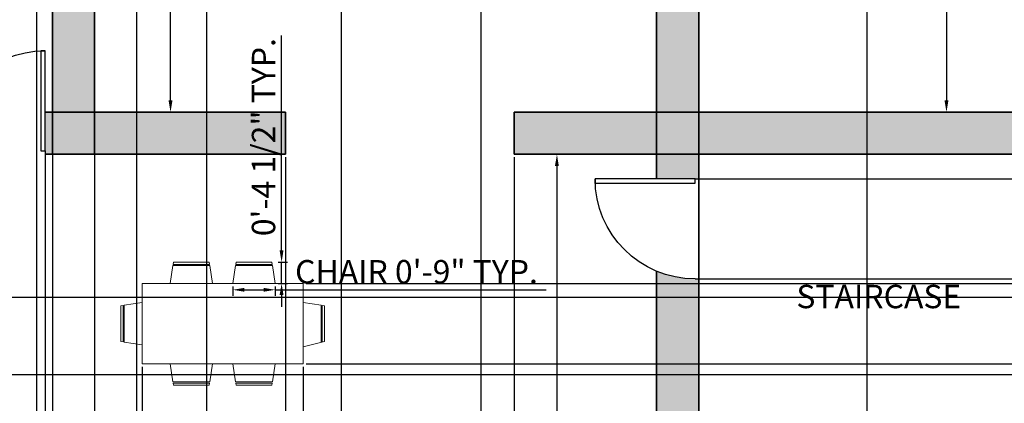
# Model space of a CAD drawing. Units: millimetres. Extents: x 2803 to 3393, y 965 to 1464.
# Tile 4 of 6: x 2962 to 3172, y 1236 to 1318. Entities that reach past the tile are written whole.
import ezdxf

# ---------------------------------------------------------------- set-up
doc = ezdxf.new("R2010")
doc.units = ezdxf.units.MM
for name, color, linetype, lineweight in [('A-ANNO-DIMS', 150, 'Continuous', 18), ('A-AREA-IDEN', 200, 'Continuous', 25), ('A-WALL-PATT', 2, 'Continuous', 13), ('doors', 10, 'Continuous', 25), ('furniture', 70, 'Continuous', 18), ('walls', 2, 'Continuous', 35)]:
    doc.layers.add(name, color=color, linetype=linetype, lineweight=lineweight)
doc.styles.get("Standard").update_dxf_attribs({"font": 'arial.ttf'})
doc.dimstyles.new('ISO-25', dxfattribs={"dimtxt": 5, "dimasz": 2.5, "dimexe": 1.25, "dimexo": 0.625, "dimtad": 1, "dimdec": 0, "dimlunit": 3, "dimtxsty": 'Standard', "dimcen": 2.5, "dimadec": 0, "dimazin": 0, "dimtfac": 1, "dimtdec": 0, "dimtmove": 0, "dimatfit": 3, "dimfxl": 1, "dimarcsym": 0})

# ---------------------------------------------------------------- blocks, each defined once
blk = doc.blocks.new('*U2')
for p, q in [((0, 0), (0, -6)), ((40, 0), (40, -6))]:
    blk.add_line(p, q)
blk.add_lwpolyline([(0, 0), (0, 40), (1.75, 40), (1.75, 0)], close=True)
blk.add_arc((0, 0), 40, 0, 90)
blk = doc.blocks.new('*D15')
at = {"layer": 'A-ANNO-DIMS', "color": 0, "lineweight": -2, "transparency": 16777216}
for p, q in [((2986.56, 1418.56), (2995.15, 1418.56)), ((2993.9, 1301.06), (2993.9, 1416.06)), ((2986.56, 1298.56), (2995.15, 1298.56))]:
    blk.add_line(p, q, dxfattribs=at)
at = {"layer": 'A-ANNO-DIMS', "color": 0, "transparency": 16777216}
for points in [[(2993.48, 1416.06), (2994.31, 1416.06), (2993.9, 1418.56)], [(2993.48, 1301.06), (2994.31, 1301.06), (2993.9, 1298.56)]]:
    blk.add_solid(points, dxfattribs=at)
at = {"layer": 'Defpoints', "color": 0, "transparency": 16777216}
for p in [(2985.93, 1418.56), (2993.9, 1418.56), (2985.93, 1298.56)]:
    blk.add_point(p, dxfattribs=at)
at = {"layer": 'A-ANNO-DIMS', "color": 0, "transparency": 16777216, "insert": (2990.72, 1358.56), "char_height": 5, "attachment_point": 5, "rotation": 90}
blk.add_mtext("10'", dxfattribs=at)
blk = doc.blocks.new('*D16')
at = {"layer": 'A-ANNO-DIMS', "color": 0, "lineweight": -2, "transparency": 16777216}
for p, q in [((3165.42, 1418.56), (3158.35, 1418.56)), ((3159.6, 1416.06), (3159.6, 1301.06)), ((3165.42, 1298.56), (3158.35, 1298.56))]:
    blk.add_line(p, q, dxfattribs=at)
at = {"layer": 'A-ANNO-DIMS', "color": 0, "transparency": 16777216}
for points in [[(3159.18, 1416.06), (3160.01, 1416.06), (3159.6, 1418.56)], [(3159.18, 1301.06), (3160.01, 1301.06), (3159.6, 1298.56)]]:
    blk.add_solid(points, dxfattribs=at)
at = {"layer": 'Defpoints', "color": 0, "transparency": 16777216}
for p in [(3166.04, 1418.56), (3159.6, 1298.56), (3166.04, 1298.56)]:
    blk.add_point(p, dxfattribs=at)
at = {"layer": 'A-ANNO-DIMS', "color": 0, "transparency": 16777216, "insert": (3156.42, 1358.56), "char_height": 5, "attachment_point": 5, "rotation": 90}
blk.add_mtext("10'", dxfattribs=at)
blk = doc.blocks.new('*D19')
at = {"layer": 'A-ANNO-DIMS', "color": 0, "lineweight": -2, "transparency": 16777216}
for p, q in [((3077.03, 1289.56), (3077.66, 1289.56)), ((3076.41, 1287.06), (3076.41, 1129.06)), ((3077.03, 1126.56), (3077.66, 1126.56))]:
    blk.add_line(p, q, dxfattribs=at)
at = {"layer": 'A-ANNO-DIMS', "color": 0, "transparency": 16777216}
for points in [[(3075.99, 1287.06), (3076.82, 1287.06), (3076.41, 1289.56)], [(3075.99, 1129.06), (3076.82, 1129.06), (3076.41, 1126.56)]]:
    blk.add_solid(points, dxfattribs=at)
at = {"layer": 'Defpoints', "color": 0, "transparency": 16777216}
for p in [(3076.41, 1289.56), (3076.41, 1126.56), (3076.41, 1126.56)]:
    blk.add_point(p, dxfattribs=at)
at = {"layer": 'A-ANNO-DIMS', "color": 0, "transparency": 16777216, "insert": (3073.23, 1208.06), "char_height": 5, "attachment_point": 5, "rotation": 90}
blk.add_mtext('13\'-7"', dxfattribs=at)
blk = doc.blocks.new('CHAIR-DINING')
for p, q in [((0.71, 4.54), (0.63, 4.06)), ((0.71, 4.54), (8.35, 4.54)), ((8.42, 4.06), (8.35, 4.54)), ((0.6, 3.82), (0, 0)), ((0.6, 3.82), (8.46, 3.82)), ((8.43, 4.06), (0.64, 4.06)), ((9.06, 0), (8.46, 3.82))]:
    blk.add_line(p, q)
blk = doc.blocks.new('*D33')
at = {"layer": 'A-ANNO-DIMS', "color": 0, "lineweight": -2, "transparency": 16777216}
for p, q in [((3007.19, 1261.38), (3007.19, 1259.39)), ((3009.69, 1260.64), (3013.75, 1260.64)), ((3016.25, 1261.38), (3016.25, 1259.39)), ((3016.25, 1260.64), (3074.09, 1260.64))]:
    blk.add_line(p, q, dxfattribs=at)
at = {"layer": 'A-ANNO-DIMS', "color": 0, "transparency": 16777216}
for points in [[(3009.69, 1261.06), (3009.69, 1260.23), (3007.19, 1260.64)], [(3013.75, 1261.06), (3013.75, 1260.23), (3016.25, 1260.64)]]:
    blk.add_solid(points, dxfattribs=at)
at = {"layer": 'Defpoints', "color": 0, "transparency": 16777216}
for p in [(3007.19, 1262), (3016.25, 1262), (3016.25, 1260.64)]:
    blk.add_point(p, dxfattribs=at)
at = {"layer": 'A-ANNO-DIMS', "color": 0, "transparency": 16777216, "insert": (3046.42, 1263.85), "char_height": 5, "attachment_point": 5}
blk.add_mtext('CHAIR 0\'-9" TYP.', dxfattribs=at)
blk = doc.blocks.new('*D34')
at = {"layer": 'A-ANNO-DIMS', "color": 0, "lineweight": -2, "transparency": 16777216}
for p, q in [((3017.61, 1269.04), (3017.61, 1314.92)), ((3016.87, 1266.54), (3018.86, 1266.54)), ((3017.61, 1262), (3017.61, 1266.54)), ((3016.87, 1262), (3018.86, 1262)), ((3017.61, 1259.5), (3017.61, 1257))]:
    blk.add_line(p, q, dxfattribs=at)
at = {"layer": 'A-ANNO-DIMS', "color": 0, "transparency": 16777216}
for points in [[(3017.19, 1269.04), (3018.02, 1269.04), (3017.61, 1266.54)], [(3017.19, 1259.5), (3018.02, 1259.5), (3017.61, 1262)]]:
    blk.add_solid(points, dxfattribs=at)
at = {"layer": 'Defpoints', "color": 0, "transparency": 16777216}
for p in [(3016.25, 1266.54), (3017.61, 1266.54), (3016.25, 1262)]:
    blk.add_point(p, dxfattribs=at)
at = {"layer": 'A-ANNO-DIMS', "color": 0, "transparency": 16777216, "insert": (3014.4, 1293.23), "char_height": 5, "attachment_point": 5, "rotation": 90}
blk.add_mtext('0\'-4 1/2" TYP.', dxfattribs=at)
blk = doc.blocks.new('*D43')
at = {"layer": 'A-ANNO-DIMS', "color": 0, "lineweight": -2, "transparency": 16777216}
for p, q in [((3106.68, 1230.24), (3106.68, 1454.97)), ((3109.18, 1453.72), (3140.18, 1453.72)), ((3142.68, 1230.24), (3142.68, 1454.97))]:
    blk.add_line(p, q, dxfattribs=at)
at = {"layer": 'A-ANNO-DIMS', "color": 0, "transparency": 16777216}
for points in [[(3109.18, 1454.14), (3109.18, 1453.31), (3106.68, 1453.72)], [(3140.18, 1454.14), (3140.18, 1453.31), (3142.68, 1453.72)]]:
    blk.add_solid(points, dxfattribs=at)
at = {"layer": 'Defpoints', "color": 0, "transparency": 16777216}
for p in [(3142.68, 1453.72), (3106.68, 1229.61), (3142.68, 1229.61)]:
    blk.add_point(p, dxfattribs=at)
at = {"layer": 'A-ANNO-DIMS', "color": 0, "transparency": 16777216, "insert": (3124.68, 1456.9), "char_height": 5, "attachment_point": 5}
blk.add_mtext('3\'-0"', dxfattribs=at)
blk = doc.blocks.new('*D45')
at = {"layer": 'A-ANNO-DIMS', "color": 0, "lineweight": -2, "transparency": 16777216}
for p, q in [((3200.68, 1297.94), (3200.68, 968.15)), ((3106.68, 1288.94), (3106.68, 968.15)), ((3109.18, 969.4), (3198.18, 969.4))]:
    blk.add_line(p, q, dxfattribs=at)
at = {"layer": 'A-ANNO-DIMS', "color": 0, "transparency": 16777216}
for points in [[(3109.18, 969.82), (3109.18, 968.99), (3106.68, 969.4)], [(3198.18, 969.82), (3198.18, 968.99), (3200.68, 969.4)]]:
    blk.add_solid(points, dxfattribs=at)
at = {"layer": 'Defpoints', "color": 0, "transparency": 16777216}
for p in [(3200.68, 1298.56), (3106.68, 1289.56), (3200.68, 969.4)]:
    blk.add_point(p, dxfattribs=at)
at = {"layer": 'A-ANNO-DIMS', "color": 0, "transparency": 16777216, "insert": (3153.68, 972.58), "char_height": 5, "attachment_point": 5}
blk.add_mtext('7\'-10"', dxfattribs=at)
blk = doc.blocks.new('*D46')
at = {"layer": 'A-ANNO-DIMS', "color": 0, "lineweight": -2, "transparency": 16777216}
for p, q in [((3067.93, 1289.56), (3390.09, 1289.56)), ((3388.84, 1232.11), (3388.84, 1287.06)), ((3201.31, 1229.61), (3390.09, 1229.61))]:
    blk.add_line(p, q, dxfattribs=at)
at = {"layer": 'A-ANNO-DIMS', "color": 0, "transparency": 16777216}
for points in [[(3388.43, 1287.06), (3389.26, 1287.06), (3388.84, 1289.56)], [(3388.43, 1232.11), (3389.26, 1232.11), (3388.84, 1229.61)]]:
    blk.add_solid(points, dxfattribs=at)
at = {"layer": 'Defpoints', "color": 0, "transparency": 16777216}
for p in [(3067.31, 1289.56), (3388.84, 1289.56), (3200.68, 1229.61)]:
    blk.add_point(p, dxfattribs=at)
at = {"layer": 'A-ANNO-DIMS', "color": 0, "transparency": 16777216, "insert": (3385.67, 1259.59), "char_height": 5, "attachment_point": 5, "rotation": 90}
blk.add_mtext('5\'-0"', dxfattribs=at)
blk = doc.blocks.new('*D61')
at = {"layer": 'A-ANNO-DIMS', "color": 0, "lineweight": -2, "transparency": 16777216}
for p, q in [((3001.68, 1025.19), (3001.68, 1454.97)), ((3004.18, 1453.72), (3027.9, 1453.72)), ((3030.4, 1025.19), (3030.4, 1454.97))]:
    blk.add_line(p, q, dxfattribs=at)
at = {"layer": 'A-ANNO-DIMS', "color": 0, "transparency": 16777216}
for points in [[(3004.18, 1454.14), (3004.18, 1453.31), (3001.68, 1453.72)], [(3027.9, 1454.14), (3027.9, 1453.31), (3030.4, 1453.72)]]:
    blk.add_solid(points, dxfattribs=at)
at = {"layer": 'Defpoints', "color": 0, "transparency": 16777216}
for p in [(3030.4, 1453.72), (3001.68, 1024.56), (3030.4, 1024.56)]:
    blk.add_point(p, dxfattribs=at)
at = {"layer": 'A-ANNO-DIMS', "color": 0, "transparency": 16777216, "insert": (3016.04, 1456.93), "char_height": 5, "attachment_point": 5}
blk.add_mtext('2\'-4 1/2"', dxfattribs=at)
blk = doc.blocks.new('*D62')
at = {"layer": 'A-ANNO-DIMS', "color": 0, "lineweight": -2, "transparency": 16777216}
for p, q in [((3030.4, 1025.19), (3030.4, 1454.97)), ((3032.9, 1453.72), (3057.7, 1453.72)), ((3060.2, 1025.19), (3060.2, 1454.97))]:
    blk.add_line(p, q, dxfattribs=at)
at = {"layer": 'A-ANNO-DIMS', "color": 0, "transparency": 16777216}
for points in [[(3032.9, 1454.14), (3032.9, 1453.31), (3030.4, 1453.72)], [(3057.7, 1454.14), (3057.7, 1453.31), (3060.2, 1453.72)]]:
    blk.add_solid(points, dxfattribs=at)
at = {"layer": 'Defpoints', "color": 0, "transparency": 16777216}
for p in [(3060.2, 1453.72), (3030.4, 1024.56), (3060.2, 1024.56)]:
    blk.add_point(p, dxfattribs=at)
at = {"layer": 'A-ANNO-DIMS', "color": 0, "transparency": 16777216, "insert": (3045.3, 1456.9), "char_height": 5, "attachment_point": 5}
blk.add_mtext('2\'-6"', dxfattribs=at)
blk = doc.blocks.new('*D63')
at = {"layer": 'A-ANNO-DIMS', "color": 0, "lineweight": -2, "transparency": 16777216}
for p, q in [((2968.68, 1426.94), (2968.68, 968.15)), ((2977.68, 1426.94), (2977.68, 968.15)), ((2971.18, 969.4), (2975.18, 969.4)), ((2977.68, 969.4), (2994.73, 969.4))]:
    blk.add_line(p, q, dxfattribs=at)
at = {"layer": 'A-ANNO-DIMS', "color": 0, "transparency": 16777216}
for points in [[(2971.18, 969.82), (2971.18, 968.99), (2968.68, 969.4)], [(2975.18, 969.82), (2975.18, 968.99), (2977.68, 969.4)]]:
    blk.add_solid(points, dxfattribs=at)
at = {"layer": 'Defpoints', "color": 0, "transparency": 16777216}
for p in [(2968.68, 1427.56), (2977.68, 1427.56), (2977.68, 969.4)]:
    blk.add_point(p, dxfattribs=at)
at = {"layer": 'A-ANNO-DIMS', "color": 0, "transparency": 16777216, "insert": (2987.45, 972.58), "char_height": 5, "attachment_point": 5}
blk.add_mtext('0\'-9"', dxfattribs=at)
blk = doc.blocks.new('*D64')
at = {"layer": 'A-ANNO-DIMS', "color": 0, "lineweight": -2, "transparency": 16777216}
for p, q in [((3018.47, 1288.94), (3018.47, 968.15)), ((3067.31, 1288.94), (3067.31, 968.15)), ((3020.97, 969.4), (3064.81, 969.4))]:
    blk.add_line(p, q, dxfattribs=at)
at = {"layer": 'A-ANNO-DIMS', "color": 0, "transparency": 16777216}
for points in [[(3020.97, 969.82), (3020.97, 968.99), (3018.47, 969.4)], [(3064.81, 969.82), (3064.81, 968.99), (3067.31, 969.4)]]:
    blk.add_solid(points, dxfattribs=at)
at = {"layer": 'Defpoints', "color": 0, "transparency": 16777216}
for p in [(3018.47, 1289.56), (3067.31, 1289.56), (3067.31, 969.4)]:
    blk.add_point(p, dxfattribs=at)
at = {"layer": 'A-ANNO-DIMS', "color": 0, "transparency": 16777216, "insert": (3042.89, 972.54), "char_height": 5, "attachment_point": 5}
blk.add_mtext('4\'-1"', dxfattribs=at)
blk = doc.blocks.new('*D65')
at = {"layer": 'A-ANNO-DIMS', "color": 0, "lineweight": -2, "transparency": 16777216}
for p, q in [((2987.84, 1244.19), (2987.84, 968.15)), ((3022.23, 1244.19), (3022.23, 968.15)), ((2990.34, 969.4), (3019.73, 969.4))]:
    blk.add_line(p, q, dxfattribs=at)
at = {"layer": 'A-ANNO-DIMS', "color": 0, "transparency": 16777216}
for points in [[(2990.34, 969.82), (2990.34, 968.99), (2987.84, 969.4)], [(3019.73, 969.82), (3019.73, 968.99), (3022.23, 969.4)]]:
    blk.add_solid(points, dxfattribs=at)
at = {"layer": 'Defpoints', "color": 0, "transparency": 16777216}
for p in [(2987.84, 1244.81), (3022.23, 1244.81), (3022.23, 969.4)]:
    blk.add_point(p, dxfattribs=at)
at = {"layer": 'A-ANNO-DIMS', "color": 0, "transparency": 16777216, "insert": (3005.03, 972.61), "char_height": 5, "attachment_point": 5}
blk.add_mtext('2\'-10 1/2"', dxfattribs=at)
blk = doc.blocks.new('*D66')
at = {"layer": 'A-ANNO-DIMS', "color": 0, "lineweight": -2, "transparency": 16777216}
for p, q in [((3022.85, 1262), (3390.09, 1262)), ((3388.84, 1247.31), (3388.84, 1259.5)), ((3022.85, 1244.81), (3390.09, 1244.81))]:
    blk.add_line(p, q, dxfattribs=at)
at = {"layer": 'A-ANNO-DIMS', "color": 0, "transparency": 16777216}
for points in [[(3388.43, 1259.5), (3389.26, 1259.5), (3388.84, 1262)], [(3388.43, 1247.31), (3389.26, 1247.31), (3388.84, 1244.81)]]:
    blk.add_solid(points, dxfattribs=at)
at = {"layer": 'Defpoints', "color": 0, "transparency": 16777216}
for p in [(3022.23, 1262), (3388.84, 1262), (3022.23, 1244.81)]:
    blk.add_point(p, dxfattribs=at)
at = {"layer": 'A-ANNO-DIMS', "color": 0, "transparency": 16777216, "insert": (3385.67, 1253.41), "char_height": 5, "attachment_point": 5, "rotation": 90}
blk.add_mtext('1\'-5"', dxfattribs=at)
blk = doc.blocks.new('*D67')
at = {"layer": 'A-ANNO-DIMS', "color": 0, "lineweight": -2, "transparency": 16777216}
for p, q in [((2945.75, 1288.94), (2945.75, 968.15)), ((2967.14, 1288.94), (2967.14, 968.15)), ((2948.25, 969.4), (2964.64, 969.4)), ((2967.14, 969.4), (2995.36, 969.4))]:
    blk.add_line(p, q, dxfattribs=at)
at = {"layer": 'A-ANNO-DIMS', "color": 0, "transparency": 16777216}
for points in [[(2948.25, 969.82), (2948.25, 968.99), (2945.75, 969.4)], [(2964.64, 969.82), (2964.64, 968.99), (2967.14, 969.4)]]:
    blk.add_solid(points, dxfattribs=at)
at = {"layer": 'Defpoints', "color": 0, "transparency": 16777216}
for p in [(2945.75, 1289.56), (2967.14, 1289.56), (2967.14, 969.4)]:
    blk.add_point(p, dxfattribs=at)
at = {"layer": 'A-ANNO-DIMS', "color": 0, "transparency": 16777216, "insert": (2982.5, 972.61), "char_height": 5, "attachment_point": 5}
blk.add_mtext('1\'-9 1/2"', dxfattribs=at)
blk = doc.blocks.new('*D68')
at = {"layer": 'A-ANNO-DIMS', "color": 0, "lineweight": -2, "transparency": 16777216}
for p, q in [((3388.84, 1259.07), (3388.84, 1287.29)), ((2942.31, 1259.07), (3390.09, 1259.07)), ((3388.84, 1245.09), (3388.84, 1256.57)), ((2942.31, 1242.59), (3390.09, 1242.59))]:
    blk.add_line(p, q, dxfattribs=at)
at = {"layer": 'A-ANNO-DIMS', "color": 0, "transparency": 16777216}
for points in [[(3388.43, 1256.57), (3389.26, 1256.57), (3388.84, 1259.07)], [(3388.43, 1245.09), (3389.26, 1245.09), (3388.84, 1242.59)]]:
    blk.add_solid(points, dxfattribs=at)
at = {"layer": 'Defpoints', "color": 0, "transparency": 16777216}
for p in [(2941.68, 1259.07), (3388.84, 1259.07), (2941.68, 1242.59)]:
    blk.add_point(p, dxfattribs=at)
at = {"layer": 'A-ANNO-DIMS', "color": 0, "transparency": 16777216, "insert": (3385.63, 1274.43), "char_height": 5, "attachment_point": 5, "rotation": 90}
blk.add_mtext('1\'-4 1/2"', dxfattribs=at)
blk = doc.blocks.new('*D70')
at = {"layer": 'A-ANNO-DIMS', "color": 0, "lineweight": -2, "transparency": 16777216}
for p, q in [((2965.38, 1175.19), (2965.38, 1454.97)), ((2967.88, 1453.72), (2984.19, 1453.72)), ((2986.69, 1175.19), (2986.69, 1454.97)), ((2986.69, 1453.72), (3014.92, 1453.72))]:
    blk.add_line(p, q, dxfattribs=at)
at = {"layer": 'A-ANNO-DIMS', "color": 0, "transparency": 16777216}
for points in [[(2967.88, 1454.14), (2967.88, 1453.31), (2965.38, 1453.72)], [(2984.19, 1454.14), (2984.19, 1453.31), (2986.69, 1453.72)]]:
    blk.add_solid(points, dxfattribs=at)
at = {"layer": 'Defpoints', "color": 0, "transparency": 16777216}
for p in [(2986.69, 1453.72), (2965.38, 1174.56), (2986.69, 1174.56)]:
    blk.add_point(p, dxfattribs=at)
at = {"layer": 'A-ANNO-DIMS', "color": 0, "transparency": 16777216, "insert": (3002.06, 1456.93), "char_height": 5, "attachment_point": 5}
blk.add_mtext('1\'-9 1/2"', dxfattribs=at)
blk = doc.blocks.new('*D72')
at = {"layer": 'A-ANNO-DIMS', "color": 0, "lineweight": -2, "transparency": 16777216}
for p, q in [((3388.84, 1284.35), (3388.84, 1312.57)), ((3107.31, 1284.35), (3390.09, 1284.35)), ((3388.84, 1265.46), (3388.84, 1281.85)), ((3107.31, 1262.96), (3390.09, 1262.96))]:
    blk.add_line(p, q, dxfattribs=at)
at = {"layer": 'A-ANNO-DIMS', "color": 0, "transparency": 16777216}
for points in [[(3388.43, 1281.85), (3389.26, 1281.85), (3388.84, 1284.35)], [(3388.43, 1265.46), (3389.26, 1265.46), (3388.84, 1262.96)]]:
    blk.add_solid(points, dxfattribs=at)
at = {"layer": 'Defpoints', "color": 0, "transparency": 16777216}
for p in [(3106.68, 1284.35), (3388.84, 1284.35), (3106.68, 1262.96)]:
    blk.add_point(p, dxfattribs=at)
at = {"layer": 'A-ANNO-DIMS', "color": 0, "transparency": 16777216, "insert": (3385.63, 1299.71), "char_height": 5, "attachment_point": 5, "rotation": 90}
blk.add_mtext('1\'-9 1/2"', dxfattribs=at)
blk = doc.blocks.new('*D74')
at = {"layer": 'A-ANNO-DIMS', "color": 0, "lineweight": -2, "transparency": 16777216}
for p, q in [((3388.84, 1232.56), (3388.84, 1260.78)), ((2869.11, 1232.56), (3390.09, 1232.56)), ((3388.84, 1220.39), (3388.84, 1230.06)), ((2933.31, 1217.89), (3390.09, 1217.89))]:
    blk.add_line(p, q, dxfattribs=at)
at = {"layer": 'A-ANNO-DIMS', "color": 0, "transparency": 16777216}
for points in [[(3388.43, 1230.06), (3389.26, 1230.06), (3388.84, 1232.56)], [(3388.43, 1220.39), (3389.26, 1220.39), (3388.84, 1217.89)]]:
    blk.add_solid(points, dxfattribs=at)
at = {"layer": 'Defpoints', "color": 0, "transparency": 16777216}
for p in [(2868.49, 1232.56), (3388.84, 1232.56), (2932.68, 1217.89)]:
    blk.add_point(p, dxfattribs=at)
at = {"layer": 'A-ANNO-DIMS', "color": 0, "transparency": 16777216, "insert": (3385.63, 1247.92), "char_height": 5, "attachment_point": 5, "rotation": 90}
blk.add_mtext('1\'-2 1/2"', dxfattribs=at)

msp = doc.modelspace()

# ---------------------------------------------------------------- hatches: boundary and pattern name
at = {"layer": 'A-WALL-PATT'}
h = msp.add_hatch(color=256, dxfattribs=at)
h.dxf.hatch_style = 1
h.paths.add_polyline_path([(2968.68, 1427.56), (2919.98, 1427.56), (2919.98, 1418.56), (2968.68, 1418.56)])
h.paths.add_polyline_path([(2977.68, 1427.56), (2968.68, 1427.56), (2968.68, 1418.56), (2977.68, 1418.56)])
h.paths.add_polyline_path([(2977.68, 1418.56), (2968.68, 1418.56), (2968.68, 1298.56), (2977.68, 1298.56)])
h.paths.add_polyline_path([(3021.74, 1427.56), (2977.68, 1427.56), (2977.68, 1418.56), (3021.74, 1418.56)])
h.paths.add_polyline_path([(2881.7, 1427.56), (2848.68, 1427.56), (2848.68, 1418.56), (2881.7, 1418.56)])
h.paths.add_polyline_path([(2848.68, 1427.56), (2839.68, 1427.56), (2839.68, 1418.56), (2848.68, 1418.56)])
h.paths.add_polyline_path([(2848.68, 1418.56), (2839.68, 1418.56), (2839.68, 1298.56), (2848.68, 1298.56)])
h.paths.add_polyline_path([(2932.68, 1298.56), (2848.68, 1298.56), (2848.68, 1289.56), (2932.68, 1289.56)])
h.paths.add_polyline_path([(2848.68, 1298.56), (2839.68, 1298.56), (2839.68, 1289.56), (2848.68, 1289.56)])
h.paths.add_polyline_path([(2848.68, 1289.56), (2839.68, 1289.56), (2839.68, 1280.88), (2848.68, 1280.88)])
h.paths.add_polyline_path([(2848.68, 1252.94), (2839.68, 1252.94), (2839.68, 1241.56), (2848.68, 1241.56)])
h.paths.add_polyline_path([(2848.68, 1241.56), (2839.68, 1241.56), (2839.68, 1232.56), (2848.68, 1232.56)])
h.paths.add_polyline_path([(2932.68, 1241.56), (2848.68, 1241.56), (2848.68, 1232.56), (2932.68, 1232.56)])
h.paths.add_polyline_path([(2941.68, 1241.56), (2932.68, 1241.56), (2932.68, 1232.56), (2941.68, 1232.56)])
h.paths.add_polyline_path([(2941.68, 1289.56), (2932.68, 1289.56), (2932.68, 1257.22, -0.114666), (2939.92, 1259.03), (2941.68, 1259.07)])
h.paths.add_polyline_path([(2941.68, 1298.56), (2932.68, 1298.56), (2932.68, 1289.56), (2941.68, 1289.56)])
h.paths.add_polyline_path([(2947.42, 1298.56), (2941.68, 1298.56), (2941.68, 1289.56), (2945.75, 1289.56), (2945.75, 1290.29, -0.099582)])
h.paths.add_polyline_path([(2977.68, 1298.56), (2968.68, 1298.56), (2968.68, 1289.56), (2977.68, 1289.56)])
h.paths.add_polyline_path([(3018.47, 1298.56), (2977.68, 1298.56), (2977.68, 1289.56), (3018.47, 1289.56)])
h.paths.add_polyline_path([(3097.68, 1298.56), (3067.31, 1298.56), (3067.31, 1289.56), (3097.68, 1289.56)])
h.paths.add_polyline_path([(3106.68, 1298.56), (3097.68, 1298.56), (3097.68, 1289.56), (3106.68, 1289.56)])
h.paths.add_polyline_path([(3200.68, 1298.56), (3106.68, 1298.56), (3106.68, 1289.56), (3200.68, 1289.56)])
h.paths.add_polyline_path([(3209.68, 1298.56), (3200.68, 1298.56), (3200.68, 1289.56), (3209.68, 1289.56)])
h.paths.add_polyline_path([(3209.68, 1289.56), (3200.68, 1289.56), (3200.68, 1270.22), (3209.68, 1270.22)])
h.paths.add_polyline_path([(3106.68, 1418.56), (3097.68, 1418.56), (3097.68, 1298.56), (3106.68, 1298.56)])
h.paths.add_polyline_path([(3106.68, 1427.56), (3097.68, 1427.56), (3097.68, 1418.56), (3106.68, 1418.56)])
h.paths.add_polyline_path([(3097.68, 1427.56), (3058.94, 1427.56), (3058.94, 1418.56), (3097.68, 1418.56)])
h.paths.add_polyline_path([(3353.68, 1427.56), (3106.68, 1427.56), (3106.68, 1418.56), (3353.68, 1418.56)])
h.paths.add_polyline_path([(3362.68, 1427.56), (3353.68, 1427.56), (3353.68, 1418.56), (3362.68, 1418.56)])
h.paths.add_polyline_path([(3362.68, 1418.56), (3353.68, 1418.56), (3353.68, 1064.56), (3362.68, 1064.56)])
h.paths.add_polyline_path([(3362.68, 1064.56), (3353.68, 1064.56), (3353.68, 1055.56), (3362.68, 1055.56)])
h.paths.add_polyline_path([(3362.68, 1055.56), (3353.68, 1055.56), (3353.68, 995.56), (3362.68, 995.56)])
h.paths.add_polyline_path([(3353.68, 1064.56), (3209.68, 1064.56), (3209.68, 1055.56), (3353.68, 1055.56)])
h.paths.add_polyline_path([(3200.68, 1064.56), (3106.68, 1064.56), (3106.68, 1055.56), (3200.68, 1055.56)])
h.paths.add_polyline_path([(3209.68, 1064.56), (3200.68, 1064.56), (3200.68, 1055.56), (3209.68, 1055.56)])
h.paths.add_polyline_path([(3209.68, 1229.61), (3200.68, 1229.61), (3200.68, 1064.56), (3209.68, 1064.56)])
h.paths.add_polyline_path([(3106.68, 1117.56), (3097.68, 1117.56), (3097.68, 1064.56), (3106.68, 1064.56)])
h.paths.add_polyline_path([(3106.68, 1126.56), (3097.68, 1126.56), (3097.68, 1117.56), (3106.68, 1117.56)])
h.paths.add_polyline_path([(3097.68, 1126.56), (3001.68, 1126.56), (3001.68, 1117.56), (3097.68, 1117.56)])
h.paths.add_polyline_path([(3001.68, 1165.56), (2992.68, 1165.56), (2992.68, 1126.56), (3001.68, 1126.56)])
h.paths.add_polyline_path([(3001.68, 1174.56), (2992.68, 1174.56), (2992.68, 1165.56), (3001.68, 1165.56)])
h.paths.add_polyline_path([(2992.68, 1174.56), (2986.69, 1174.56), (2986.69, 1165.56), (2992.68, 1165.56)])
h.paths.add_polyline_path([(3001.68, 1126.56), (2992.68, 1126.56), (2992.68, 1117.56), (3001.68, 1117.56)])
h.paths.add_polyline_path([(3001.68, 1117.56), (2992.68, 1117.56), (2992.68, 1112.21), (2994.15, 1112.23), (3001.68, 1112.37)])
h.paths.add_polyline_path([(3001.68, 1033.56), (2992.68, 1033.56), (2992.68, 1024.56), (3001.68, 1024.56)])
h.paths.add_polyline_path([(3001.68, 1097.58, -0.114732), (2994.45, 1095.76), (2992.68, 1095.73), (2992.68, 1033.56), (3001.68, 1033.56)])
h.paths.add_polyline_path([(3030.4, 1033.56), (3001.68, 1033.56), (3001.68, 1024.56), (3030.4, 1024.56)])
h.paths.add_polyline_path([(3097.68, 1033.56), (3060.2, 1033.56), (3060.2, 1024.56), (3097.68, 1024.56)])
h.paths.add_polyline_path([(3106.68, 1033.56), (3097.68, 1033.56), (3097.68, 1024.56), (3106.68, 1024.56)])
h.paths.add_polyline_path([(3106.68, 1055.56), (3097.68, 1055.56), (3097.68, 1033.56), (3106.68, 1033.56)])
h.paths.add_polyline_path([(3106.68, 1064.56), (3097.68, 1064.56), (3097.68, 1055.56), (3106.68, 1055.56)])
h.paths.add_polyline_path([(2992.68, 1033.56), (2848.68, 1033.56), (2848.68, 1024.56), (2992.68, 1024.56)])
h.paths.add_polyline_path([(2848.68, 1033.56), (2839.68, 1033.56), (2839.68, 1024.56), (2848.68, 1024.56)])
h.paths.add_polyline_path([(2848.68, 1070.54), (2839.68, 1070.54), (2839.68, 1033.56), (2848.68, 1033.56)])
h.paths.add_polyline_path([(2848.68, 1165.56), (2839.68, 1165.56), (2839.68, 1114.52), (2848.68, 1114.52)])
h.paths.add_polyline_path([(2848.68, 1174.56), (2839.68, 1174.56), (2839.68, 1165.56), (2848.68, 1165.56)])
h.paths.add_polyline_path([(2932.68, 1174.56), (2848.68, 1174.56), (2848.68, 1165.56), (2932.68, 1165.56)])
h.paths.add_polyline_path([(2941.68, 1174.56), (2932.68, 1174.56), (2932.68, 1165.56), (2941.68, 1165.56)])
h.paths.add_polyline_path([(2965.38, 1174.56), (2941.68, 1174.56), (2941.68, 1165.56), (2968.2, 1165.56, -0.111634)])
h.paths.add_polyline_path([(2848.68, 1193.13), (2839.68, 1193.13), (2839.68, 1174.56), (2848.68, 1174.56)])
h.paths.add_polyline_path([(2848.68, 1232.56), (2839.68, 1232.56), (2839.68, 1221.86), (2848.68, 1221.86)])
h.paths.add_polyline_path([(2941.68, 1232.56), (2932.68, 1232.56), (2932.68, 1191.24, -0.132111), (2940.91, 1193.6), (2941.68, 1193.62)])
h.paths.add_polyline_path([(3106.68, 1262.96), (3105.94, 1262.96, -0.099353), (3097.68, 1264.61), (3097.68, 1126.56), (3106.68, 1126.56)])
h = msp.add_hatch(color=256, dxfattribs=at)
h.dxf.hatch_style = 1
h.paths.add_polyline_path([(3106.68, 1289.56), (3097.68, 1289.56), (3097.68, 1284.35), (3105.94, 1284.35), (3106.68, 1284.35)])
h.paths.add_polyline_path([(2968.68, 1298.56), (2967.14, 1298.56), (2967.14, 1290.29), (2967.14, 1289.56), (2968.68, 1289.56)])

# ---------------------------------------------------------------- linework, layer by layer
at = {"layer": 'furniture'}
for p, q in [((3022.23, 1262), (2987.84, 1262)), ((2987.84, 1262), (2987.84, 1244.81)), ((3022.23, 1244.81), (3022.23, 1262)), ((3026.05, 1257.34), (3022.22, 1257.94)), ((3026.05, 1257.34), (3026.05, 1249.41)), ((3026.76, 1257.23), (3026.29, 1257.3)), ((3026.29, 1249.47), (3026.29, 1257.3)), ((3026.76, 1257.23), (3026.76, 1249.59)), ((3026.76, 1249.59), (3022.23, 1248.45)), ((3026.05, 1249.47), (3026.76, 1249.59)), ((2987.84, 1244.81), (3022.23, 1244.81))]:
    msp.add_line(p, q, dxfattribs=at)
at = {"layer": 'walls'}
for p, q in [((2968.68, 1427.56), (2968.68, 1289.56)), ((2977.68, 1427.56), (2977.68, 1289.56)), ((3097.68, 1427.56), (3097.68, 1284.35)), ((3106.68, 1427.56), (3106.68, 1284.35)), ((2967.14, 1298.56), (3018.47, 1298.56)), ((3018.47, 1298.56), (3018.47, 1289.56)), ((3067.31, 1298.56), (3067.31, 1289.56)), ((3067.31, 1298.56), (3106.68, 1298.56)), ((3106.68, 1298.56), (3209.68, 1298.56)), ((2967.14, 1289.56), (3018.47, 1289.56)), ((3067.31, 1289.56), (3106.68, 1289.56)), ((3106.68, 1289.56), (3209.68, 1289.56)), ((3097.68, 1264.61), (3097.68, 1024.56)), ((3106.68, 1262.96), (3106.68, 1024.56))]:
    msp.add_line(p, q, dxfattribs=at)

# ---------------------------------------------------------------- block references
at = {"layer": 'doors', "xscale": -0.534749261424752, "yscale": 0.534749261424752, "zscale": 0.534749261424752}
msp.add_blockref('*U2', (2967.14, 1290.29), dxfattribs=at)
at = {"layer": 'doors', "xscale": -0.534749261424752, "yscale": 0.534749261424752, "zscale": 0.534749261424752, "rotation": 90}
msp.add_blockref('*U2', (3105.94, 1284.35), dxfattribs=at)
at = {"layer": 'furniture'}
for p in [(2993.82, 1262), (3007.19, 1262)]:
    msp.add_blockref('CHAIR-DINING', p, dxfattribs=at)
at = {"layer": 'furniture', "extrusion": (0, 0, -1), "zscale": -1}
for p, rotation in [((-2987.84, 1257.94), 270), ((-2993.82, 1244.81), 180), ((-3007.19, 1244.81), 180)]:
    msp.add_blockref('CHAIR-DINING', p, dxfattribs=dict(at, rotation=rotation))

# ---------------------------------------------------------------- texts
at = {"layer": 'A-AREA-IDEN', "insert": (3127.54, 1261.71), "char_height": 5, "attachment_point": 1}
msp.add_mtext_dynamic_manual_height_columns('STAIRCASE', width=62.415, gutter_width=12.5, heights=[0], dxfattribs=at)

# ---------------------------------------------------------------- dimensions: what is measured, and where the dimension line sits
at = {"layer": 'A-ANNO-DIMS'}
for base, p1, p2, picture, middle in [((2986.69, 1453.72), (2965.38, 1174.56), (2986.69, 1174.56), '*D70', (3002.06, 1456.93)), ((3030.4, 1453.72), (3001.68, 1024.56), (3030.4, 1024.56), '*D61', (3016.04, 1456.93)), ((3060.2, 1453.72), (3030.4, 1024.56), (3060.2, 1024.56), '*D62', (3045.3, 1456.9)), ((3142.68, 1453.72), (3106.68, 1229.61), (3142.68, 1229.61), '*D43', (3124.68, 1456.9)), ((2977.68, 969.4), (2968.68, 1427.56), (2977.68, 1427.56), '*D63', (2987.45, 972.58)), ((3200.68, 969.4), (3106.68, 1289.56), (3200.68, 1298.56), '*D45', (3153.68, 972.58)), ((2967.14, 969.4), (2945.75, 1289.56), (2967.14, 1289.56), '*D67', (2982.5, 972.61)), ((3067.31, 969.4), (3018.47, 1289.56), (3067.31, 1289.56), '*D64', (3042.89, 972.54)), ((3022.23, 969.4), (2987.84, 1244.81), (3022.23, 1244.81), '*D65', (3005.03, 972.61))]:
    dim = msp.add_linear_dim(base=base, p1=p1, p2=p2, dimstyle='ISO-25', override={"dimdec": 1, "dimlfac": 1, "dimrnd": 0, "dimzin": 1, "dimdsep": 46, "dimlunit": 4, "dimfrac": 2}, dxfattribs=at)
    dim.commit()
    dim.dimension.update_dxf_attribs({"geometry": picture, "text_midpoint": middle})
for base, p1, p2, override, picture, middle in [((2993.9, 1418.56), (2985.93, 1298.56), (2985.93, 1418.56), {"dimclrd": 0, "dimclre": 0, "dimclrt": 0}, '*D15', (2990.72, 1358.56)), ((3159.6, 1298.56), (3166.04, 1418.56), (3166.04, 1298.56), {"dimclrd": 0, "dimclre": 0, "dimclrt": 0}, '*D16', (3156.42, 1358.56)), ((3388.84, 1284.35), (3106.68, 1262.96), (3106.68, 1284.35), {"dimdec": 1, "dimlfac": 1, "dimrnd": 0, "dimzin": 1, "dimdsep": 46, "dimlunit": 4, "dimfrac": 2}, '*D72', (3385.63, 1299.71)), ((3388.8438, 1289.563), (3200.6838, 1229.614), (3067.3091, 1289.563), {"dimdec": 1, "dimlfac": 1, "dimrnd": 0, "dimzin": 1, "dimdsep": 46, "dimlunit": 4, "dimfrac": 2}, '*D46', (3385.6659, 1259.5885)), ((3076.41, 1126.56), (3076.41, 1289.56), (3076.41, 1126.56), {"dimclrd": 0, "dimclre": 0, "dimclrt": 0}, '*D19', (3073.23, 1208.06)), ((3388.84, 1259.07), (2941.68, 1242.59), (2941.68, 1259.07), {"dimdec": 1, "dimlfac": 1, "dimrnd": 0, "dimzin": 1, "dimdsep": 46, "dimlunit": 4, "dimfrac": 2}, '*D68', (3385.63, 1274.43)), ((3388.84, 1262), (3022.23, 1244.81), (3022.23, 1262), {"dimdec": 1, "dimlfac": 1, "dimrnd": 0, "dimzin": 1, "dimdsep": 46, "dimlunit": 4, "dimfrac": 2}, '*D66', (3385.67, 1253.41)), ((3388.84, 1232.56), (2932.68, 1217.89), (2868.49, 1232.56), {"dimdec": 1, "dimlfac": 1, "dimrnd": 0, "dimzin": 1, "dimdsep": 46, "dimlunit": 4, "dimfrac": 2}, '*D74', (3385.63, 1247.92))]:
    dim = msp.add_linear_dim(base=base, p1=p1, p2=p2, angle=90, dimstyle='ISO-25', override=override, dxfattribs=at)
    dim.commit()
    dim.dimension.update_dxf_attribs({"geometry": picture, "text_midpoint": middle})
dim = msp.add_linear_dim(base=(3017.61, 1266.54), p1=(3016.25, 1262), p2=(3016.25, 1266.54), angle=90, text='<> TYP.', dimstyle='ISO-25', override={"dimdec": 1, "dimlfac": 1, "dimrnd": 0, "dimzin": 1, "dimdsep": 46, "dimlunit": 4, "dimfrac": 2}, dxfattribs=at)
dim.commit()
dim.dimension.update_dxf_attribs({"geometry": '*D34', "text_midpoint": (3014.4, 1293.23)})
dim = msp.add_linear_dim(base=(3016.25, 1260.64), p1=(3007.19, 1262), p2=(3016.25, 1262), text='CHAIR <> TYP.', dimstyle='ISO-25', override={"dimdec": 1, "dimlfac": 1, "dimrnd": 0, "dimzin": 1, "dimdsep": 46, "dimlunit": 4, "dimfrac": 2}, dxfattribs=at)
dim.commit()
dim.dimension.update_dxf_attribs({"geometry": '*D33', "text_midpoint": (3046.42, 1263.85)})

doc.saveas('drawing.dxf')
